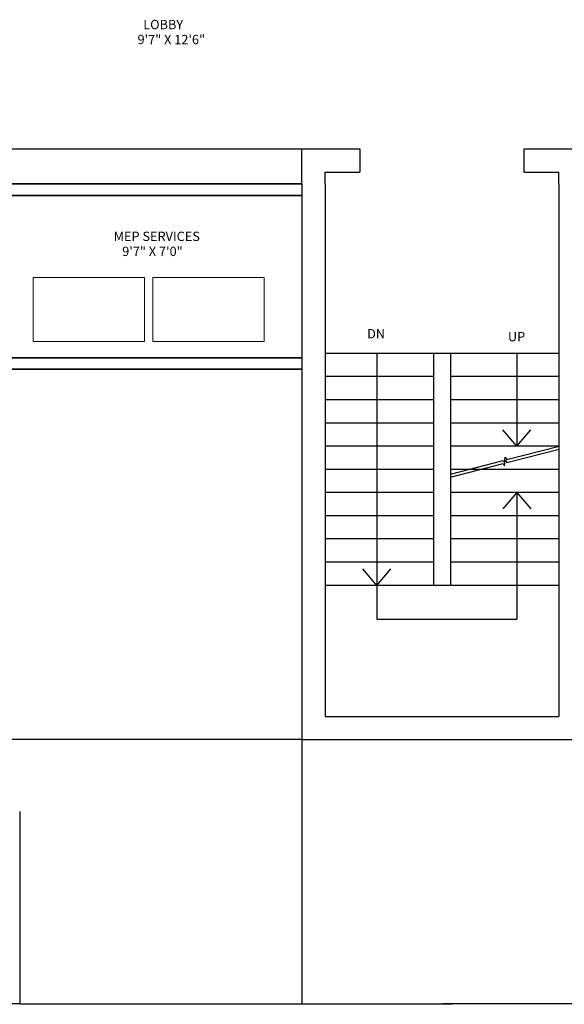
# Model space of a CAD drawing. Units: inches. Extents: x -61 to 1599, y -1316 to 257.
# Tile 31 of 204: x 545 to 826, y -1316 to -806. Entities that reach past the tile are written whole.
import ezdxf

# ---------------------------------------------------------------- set-up
doc = ezdxf.new("R2010")
doc.units = ezdxf.units.IN
doc.header["$MEASUREMENT"] = 0
for name, color, linetype, lineweight in [('A-ANNO-DIMS', 2, 'Continuous', 18), ('A-ANNO-SYMB', 1, 'Continuous', 18), ('A-AREA-IDEN', 1, 'Continuous', 18), ('A-EQPM', 9, 'Continuous', 18), ('A-FLOR-STRS', 8, 'Continuous', 25), ('WALLS', 4, 'Continuous', 35)]:
    doc.layers.add(name, color=color, linetype=linetype, lineweight=lineweight)
doc.styles.get("Standard").update_dxf_attribs({"font": 'arial.ttf'})
doc.dimstyles.get("Standard").update_dxf_attribs({"dimtxt": 0.18, "dimasz": 0.18, "dimexe": 0.18, "dimexo": 0.0625, "dimgap": 0.09, "dimtad": 0, "dimtih": 1, "dimtoh": 1, "dimdec": 0, "dimzin": 0, "dimdsep": 46, "dimlunit": 3, "dimtxsty": 'Standard', "dimcen": 0.09, "dimadec": 0, "dimazin": 0, "dimtfac": 1, "dimtdec": 0, "dimtofl": 0, "dimtmove": 0, "dimatfit": 3, "dimfxl": 1, "dimtolj": 1, "dimtzin": 0, "dimarcsym": 0})

# ---------------------------------------------------------------- blocks, each defined once
blk = doc.blocks.new('*D688')
at = {"layer": 'A-ANNO-DIMS', "color": 0, "lineweight": -2, "transparency": 16777216}
for p, q in [((14.7, -1216.01), (14.7, -1315.72)), ((544.7, -1216.01), (544.7, -1315.72)), ((14.88, -1315.54), (279.41, -1315.54)), ((544.52, -1315.54), (279.99, -1315.54))]:
    blk.add_line(p, q, dxfattribs=at)
at = {"layer": 'A-ANNO-DIMS', "color": 0, "transparency": 16777216}
for points in [[(14.88, -1315.51), (14.88, -1315.57), (14.7, -1315.54)], [(544.52, -1315.51), (544.52, -1315.57), (544.7, -1315.54)]]:
    blk.add_solid(points, dxfattribs=at)
at = {"layer": 'DEFPOINTS', "color": 0, "transparency": 16777216}
for p in [(14.7, -1215.94), (544.7, -1215.94), (544.7, -1315.54)]:
    blk.add_point(p, dxfattribs=at)
at = {"layer": 'A-ANNO-DIMS', "color": 0, "transparency": 16777216, "insert": (279.7, -1315.54), "char_height": 0.18, "attachment_point": 5}
blk.add_mtext('\\A1;530', dxfattribs=at)
blk = doc.blocks.new('*D689')
at = {"layer": 'A-ANNO-DIMS', "color": 0, "lineweight": -2, "transparency": 16777216}
for p, q in [((992.7, -1211.23), (992.7, -1315.72)), ((544.7, -1216.01), (544.7, -1315.72)), ((544.88, -1315.54), (768.41, -1315.54)), ((992.52, -1315.54), (769, -1315.54))]:
    blk.add_line(p, q, dxfattribs=at)
at = {"layer": 'A-ANNO-DIMS', "color": 0, "transparency": 16777216}
for points in [[(544.88, -1315.51), (544.88, -1315.57), (544.7, -1315.54)], [(992.52, -1315.51), (992.52, -1315.57), (992.7, -1315.54)]]:
    blk.add_solid(points, dxfattribs=at)
at = {"layer": 'DEFPOINTS', "color": 0, "transparency": 16777216}
for p in [(992.7, -1211.17), (544.7, -1215.94), (992.7, -1315.54)]:
    blk.add_point(p, dxfattribs=at)
at = {"layer": 'A-ANNO-DIMS', "color": 0, "transparency": 16777216, "insert": (768.7, -1315.54), "char_height": 0.18, "attachment_point": 5}
blk.add_mtext('\\A1;448', dxfattribs=at)
blk = doc.blocks.new('*D695')
at = {"layer": 'A-ANNO-DIMS', "color": 0, "lineweight": -2, "transparency": 16777216}
for p, q in [((690.7, -1178.86), (690.7, -1315.72)), ((835.7, -1178.86), (835.7, -1315.72)), ((690.88, -1315.54), (762.92, -1315.54)), ((835.52, -1315.54), (763.48, -1315.54))]:
    blk.add_line(p, q, dxfattribs=at)
at = {"layer": 'A-ANNO-DIMS', "color": 0, "transparency": 16777216}
for points in [[(690.88, -1315.51), (690.88, -1315.57), (690.7, -1315.54)], [(835.52, -1315.51), (835.52, -1315.57), (835.7, -1315.54)]]:
    blk.add_solid(points, dxfattribs=at)
at = {"layer": 'DEFPOINTS', "color": 0, "transparency": 16777216}
for p in [(690.7, -1178.79), (835.7, -1178.79), (835.7, -1315.54)]:
    blk.add_point(p, dxfattribs=at)
at = {"layer": 'A-ANNO-DIMS', "color": 0, "transparency": 16777216, "insert": (763.2, -1315.54), "char_height": 0.18, "attachment_point": 5}
blk.add_mtext('\\A1;145', dxfattribs=at)
blk = doc.blocks.new('*D696')
at = {"layer": 'A-ANNO-DIMS', "color": 0, "lineweight": -2, "transparency": 16777216}
for p, q in [((690.64, -873.17), (-61.08, -873.17)), ((-60.9, -873.35), (-60.9, -1025.8)), ((-60.9, -1178.61), (-60.9, -1026.16)), ((690.64, -1178.79), (-61.08, -1178.79))]:
    blk.add_line(p, q, dxfattribs=at)
at = {"layer": 'A-ANNO-DIMS', "color": 0, "transparency": 16777216}
for points in [[(-60.93, -873.35), (-60.87, -873.35), (-60.9, -873.17)], [(-60.93, -1178.61), (-60.87, -1178.61), (-60.9, -1178.79)]]:
    blk.add_solid(points, dxfattribs=at)
at = {"layer": 'DEFPOINTS', "color": 0, "transparency": 16777216}
for p in [(-60.9, -873.17), (690.7, -873.17), (690.7, -1178.79)]:
    blk.add_point(p, dxfattribs=at)
at = {"layer": 'A-ANNO-DIMS', "color": 0, "transparency": 16777216, "insert": (-60.9, -1025.98), "char_height": 0.18, "attachment_point": 5}
blk.add_mtext('\\A1;305.6', dxfattribs=at)

msp = doc.modelspace()

# ---------------------------------------------------------------- linework, layer by layer
at = {"layer": 'A-EQPM'}
for points in [[(609.2937, -972.7036), (551.6962, -972.7036), (551.6962, -939.7343), (609.2937, -939.7343)], [(671.2473, -972.7036), (613.6497, -972.7036), (613.6497, -939.7343), (671.2473, -939.7343)]]:
    msp.add_lwpolyline(points, close=True, dxfattribs=at)
at = {"layer": 'A-FLOR-STRS'}
for p, q in [((690.7028, -891.169), (690.7028, -873.169)), ((690.7028, -873.169), (702.7028, -873.169)), ((702.7028, -873.169), (720.7028, -873.169)), ((720.7028, -873.169), (720.7028, -885.169)), ((805.7028, -873.169), (823.7028, -873.169)), ((805.7028, -885.169), (805.7028, -873.169)), ((823.7028, -873.169), (835.7028, -873.169)), ((702.7028, -891.169), (702.7028, -885.169)), ((702.7028, -885.169), (720.7028, -885.169)), ((805.7028, -885.169), (823.7028, -885.169)), ((823.7028, -891.169), (823.7028, -885.169)), ((690.7028, -891.169), (690.7028, -1178.7933)), ((702.7028, -891.169), (702.7028, -1166.7933)), ((823.7028, -891.169), (823.7028, -1166.7933)), ((823.7028, -978.9562), (702.7028, -978.9562)), ((729.4357, -978.9562), (729.4357, -1116.4552)), ((758.9286, -1098.9562), (758.9286, -978.9562)), ((767.7608, -1098.9562), (767.7608, -978.9562)), ((801.973, -978.9562), (801.973, -1026.9562)), ((758.9286, -990.9562), (702.7028, -990.9562)), ((823.7028, -990.9562), (767.7608, -990.9562)), ((758.9286, -1002.9562), (702.7028, -1002.9562)), ((823.7028, -1002.9562), (767.7608, -1002.9562)), ((758.9286, -1014.9562), (702.7028, -1014.9562)), ((823.7028, -1014.9562), (767.7608, -1014.9562)), ((801.973, -1026.9562), (794.734, -1018.4774)), ((801.973, -1026.9562), (809.212, -1018.4774)), ((758.9286, -1026.9562), (702.7028, -1026.9562)), ((823.7028, -1026.9562), (767.7608, -1026.9562)), ((758.9286, -1038.9562), (702.7028, -1038.9562)), ((823.7028, -1038.9562), (767.7608, -1038.9562)), ((758.9286, -1050.9562), (702.7028, -1050.9562)), ((823.7028, -1050.9562), (767.7608, -1050.9562)), ((801.973, -1050.9562), (794.734, -1059.435)), ((801.973, -1050.9562), (801.973, -1116.4552)), ((801.973, -1050.9562), (809.212, -1059.435)), ((758.9286, -1062.9562), (702.7028, -1062.9562)), ((823.7028, -1062.9562), (767.7608, -1062.9562)), ((758.9286, -1074.9562), (702.7028, -1074.9562)), ((823.7028, -1074.9562), (767.7608, -1074.9562)), ((758.9286, -1086.9562), (702.7028, -1086.9562)), ((823.7028, -1086.9562), (767.7608, -1086.9562)), ((729.4357, -1098.9562), (722.1966, -1090.4774)), ((729.4357, -1098.9562), (736.6747, -1090.4774)), ((823.7028, -1098.9562), (702.7028, -1098.9562)), ((729.4357, -1116.4552), (801.973, -1116.4552)), ((702.7028, -1166.7933), (823.7028, -1166.7933)), ((690.7028, -1178.7933), (835.7028, -1178.7933))]:
    msp.add_line(p, q, dxfattribs=at)
for points in [[(767.5865, -1041.4006), (794.7634, -1034.4052), (795.59, -1035.611), (795.8736, -1032.701), (796.7002, -1033.9067), (823.8771, -1026.9113)], [(767.5865, -1042.9152), (794.7634, -1035.9199), (795.59, -1037.1256), (795.8736, -1034.2156), (796.7002, -1035.4213), (823.8771, -1028.426)]]:
    msp.add_lwpolyline(points, dxfattribs=at)
at = {"layer": 'WALLS'}
for p, q in [((535.7028, -891.169), (690.7028, -891.169)), ((535.7028, -897.169), (690.7028, -897.169)), ((535.7028, -981.169), (690.7028, -981.169)), ((535.7028, -987.169), (690.7028, -987.169))]:
    msp.add_line(p, q, dxfattribs=at)

# ---------------------------------------------------------------- texts
at = {"layer": 'A-ANNO-SYMB'}
for s, p in [('DN', (724.4458, -971.1637)), ('UP', (797.3094, -972.7027))]:
    msp.add_text(s, height=4.8321, dxfattribs=at).set_placement(p)
at = {"layer": 'A-AREA-IDEN'}
for s, height, p in [('  LOBBY', 4.8321, (605.6728, -811.1806)), ('9\'7" X 12\'6"', 4.832098, (605.6728, -818.9429)), ('MEP SERVICES', 4.832098, (593.3218, -920.7792)), ('   9\'7" X 7\'0"', 4.832098, (593.3218, -928.5415))]:
    msp.add_text(s, height=height, dxfattribs=at).set_placement(p)

# ---------------------------------------------------------------- dimensions: what is measured, and where the dimension line sits
at = {"layer": 'A-ANNO-DIMS'}
dim = msp.add_linear_dim(base=(-60.8972, -873.169), p1=(690.7028, -1178.7933), p2=(690.7028, -873.169), angle=90, dimstyle='Standard', override={"dimdec": 1, "dimlfac": 1, "dimrnd": 0, "dimzin": 0, "dimdsep": 46, "dimlunit": 2}, dxfattribs=at)
dim.commit()
dim.dimension.update_dxf_attribs({"geometry": '*D696', "text_midpoint": (-60.8972, -1025.9812)})
for base, p1, p2, picture, middle in [((835.7028, -1315.5446), (690.7028, -1178.7933), (835.7028, -1178.7933), '*D695', (763.2028, -1315.5446)), ((992.7028, -1315.5446), (544.7028, -1215.9446), (992.7028, -1211.169), '*D689', (768.7028, -1315.5446)), ((544.7028, -1315.5446), (14.7028, -1215.9446), (544.7028, -1215.9446), '*D688', (279.7028, -1315.5446))]:
    dim = msp.add_linear_dim(base=base, p1=p1, p2=p2, dimstyle='Standard', override={"dimdec": 0, "dimlfac": 1, "dimrnd": 0, "dimzin": 0, "dimdsep": 46, "dimlunit": 2}, dxfattribs=at)
    dim.commit()
    dim.dimension.update_dxf_attribs({"geometry": picture, "text_midpoint": middle})

doc.saveas('drawing.dxf')
